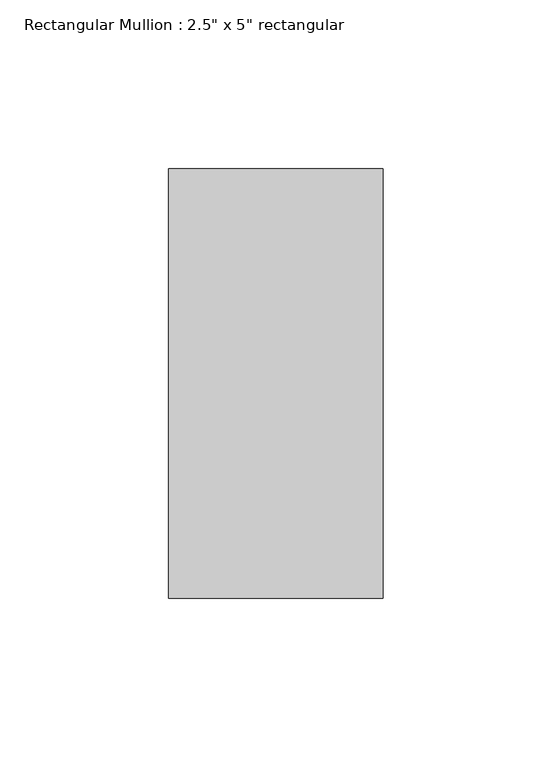
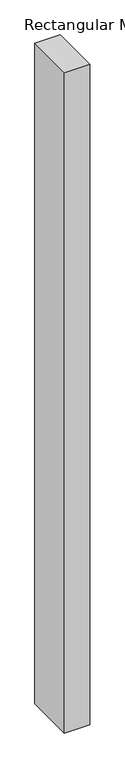
"""IFC4 building model written with IfcOpenShell, lengths in millimetres: member geometry."""

from ifc_helpers import new_model, si_unit, frame, origin, place, context, project, spatial, polyline, outline, extrude, source, transform, mapped, element, save


def member_064e5e56(model_context):
    return source(origin(), model_context, "Body", "SweptSolid", [
        extrude(outline(polyline([(31.75, 63.5), (31.75, -63.5), (-31.75, -63.5), (-31.75, 63.5), (31.75, 63.5)])), frame((0.0, 0.0, -1736.1531464), z_axis=(0.0, 0.0, 1.0), x_axis=(1.0, 0.0, 0.0)), (0.0, 0.0, 1.0), 1736.1531464),
    ])


if __name__ == "__main__":
    model = new_model("IFC4")
    model_context = context("Model", 3, world=origin())
    ifc_project = project(units=[si_unit("LENGTHUNIT", "METRE", prefix="MILLI")], contexts=[model_context])
    site = spatial("IfcSite", under=ifc_project)
    building = spatial("IfcBuilding", under=site)
    placement = place(None, origin())
    member_shape = member_064e5e56(model_context)
    element("IfcMember", 1, ObjectType="Rectangular Mullion : 2.5\" x 5\" rectangular", at=placement, inside=building, context=model_context, shape_type="MappedRepresentation", body=[
        mapped(member_shape, transform((0.0, 0.0, 0.0), x_axis=(1.0, 0.0, 0.0), y_axis=(0.0, 1.0, 0.0), z_axis=(0.0, 0.0, 1.0))),
    ])
    save(model, "model.ifc")

# Revit data of these elements
# Type "Rectangular Mullion : 2.5\" x 5\" rectangular"
#   built-in parameter 1007304 = 0.416667 (stored number, unit not read)
#   built-in parameter 1007301 = 0.104167 (stored number, unit not read)
#   built-in parameter 1007300 = 0.104167 (stored number, unit not read)
# Element 1 (IfcMember, "Rectangular Mullion : 2.5\" x 5\" rectangular")
#   Materials on its faces: "Aluminum"
# Materials
#   "Aluminum": class "Metal", colour RGB 247 247 247, transparency 0, Description = "Aluminum 6061", Cost = 0
